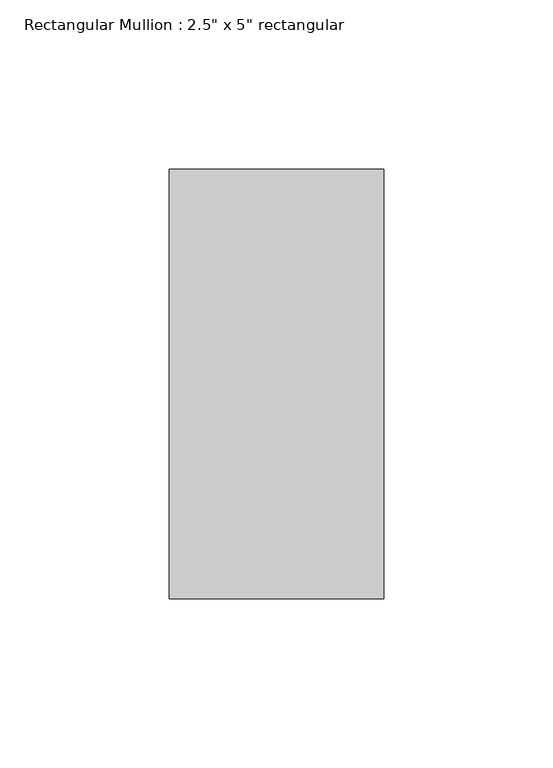
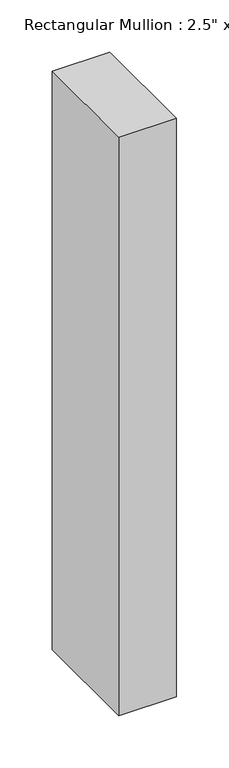
"""IFC4 building model written with IfcOpenShell, lengths in millimetres: member geometry."""

from ifc_helpers import new_model, si_unit, frame, origin, place, context, project, spatial, polyline, outline, extrude, source, transform, mapped, element, save


def member_af550d70(model_context):
    return source(origin(), model_context, "Body", "SweptSolid", [
        extrude(outline(polyline([(31.75, 63.5), (31.75, -63.5), (-31.75, -63.5), (-31.75, 63.5), (31.75, 63.5)])), frame((0.0, 0.0, -674.5371805), z_axis=(0.0, 0.0, 1.0), x_axis=(1.0, 0.0, 0.0)), (0.0, 0.0, 1.0), 674.5371805),
    ])


if __name__ == "__main__":
    model = new_model("IFC4")
    model_context = context("Model", 3, world=origin())
    ifc_project = project(units=[si_unit("LENGTHUNIT", "METRE", prefix="MILLI")], contexts=[model_context])
    site = spatial("IfcSite", under=ifc_project)
    building = spatial("IfcBuilding", under=site)
    placement = place(None, origin())
    member_shape = member_af550d70(model_context)
    element("IfcMember", 1, ObjectType="Rectangular Mullion : 2.5\" x 5\" rectangular", at=placement, inside=building, context=model_context, shape_type="MappedRepresentation", body=[
        mapped(member_shape, transform((0.0, 0.0, 0.0), x_axis=(1.0, 0.0, 0.0), y_axis=(0.0, 1.0, 0.0), z_axis=(0.0, 0.0, 1.0))),
    ])
    save(model, "model.ifc")

# Revit data of these elements
# Type "Rectangular Mullion : 2.5\" x 5\" rectangular"
#   built-in parameter 1007304 = 0.416667 (stored number, unit not read)
#   built-in parameter 1007301 = 0.104167 (stored number, unit not read)
#   built-in parameter 1007300 = 0.104167 (stored number, unit not read)
# Element 1 (IfcMember, "Rectangular Mullion : 2.5\" x 5\" rectangular")
#   Materials on its faces: "Aluminum"
# Materials
#   "Aluminum": class "Metal", colour RGB 247 247 247, transparency 0, Description = "Aluminum 6061", Cost = 0
